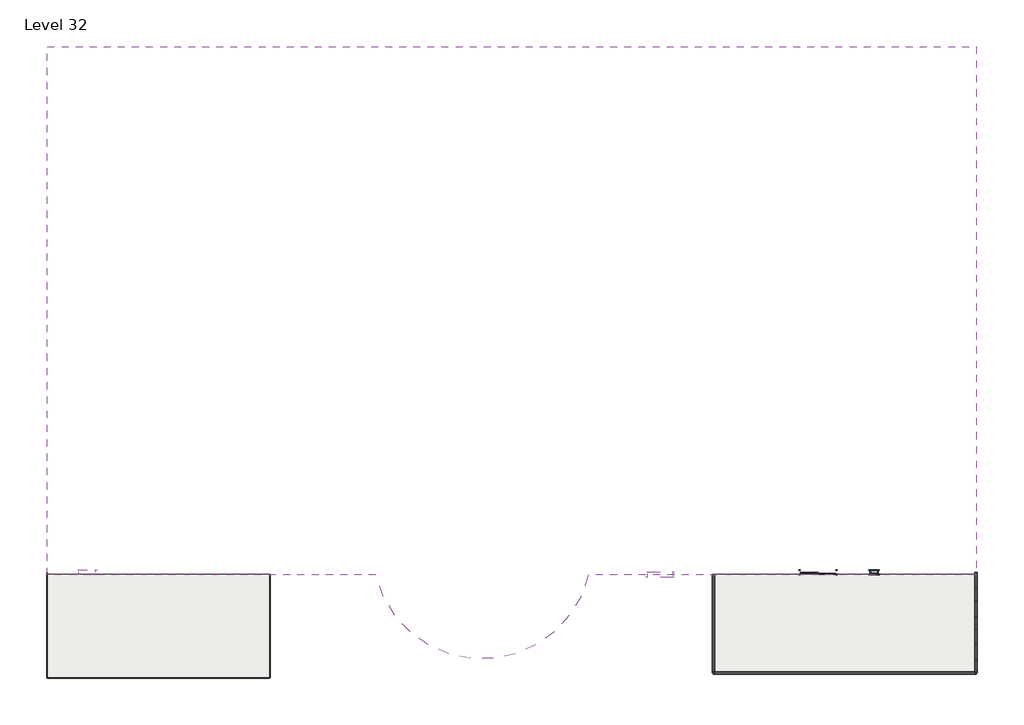
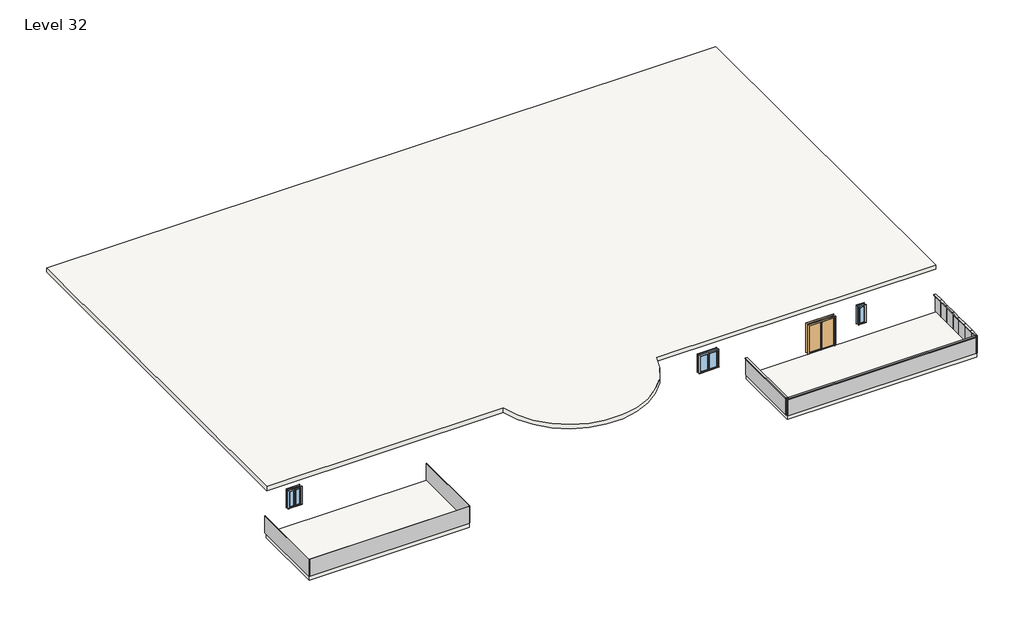
# One storey: 12 members, 12 plates, 3 slabs, 3 windows, 1 door.
"""IFC4 building model written with IfcOpenShell, lengths in millimetres."""

from ifc_helpers import new_model, si_unit, point, frame, frame_2d, origin, place, context, project, spatial, polyline, circle_curve, trimmed, segment, composite_curve, outline, extrude, transform, mapped, element, save
from components import door_076b30e0, member_bf9e663f, member_75074519, member_dd9ec6c9, member_47bfaf8a, member_aa870034, member_dcca090c, member_c1a40fae, member_a980948f, system_panel_glazed_64dbbd21, system_panel_glazed_febc6b86, system_panel_glazed_f269d4c8, system_panel_glazed_7af1c9c3, system_panel_glazed_5b6ac675, system_panel_glazed_8be6732c, system_panel_glazed_16eb27bd, system_panel_glazed_c55d8a5b, system_panel_glazed_6c4e9d17, system_panel_glazed_83eff035, window_a765b88f, window_bb17773d, window_0862ab64

model = new_model("IFC4")

# Units and contexts
model_context = context("Model", 3, world=origin())
ifc_project = project(units=[si_unit("LENGTHUNIT", "METRE", prefix="MILLI")], contexts=[model_context])

# Site, building, storey
site = spatial("IfcSite", under=ifc_project)
building = spatial("IfcBuilding", under=site)
storey = spatial("IfcBuildingStorey", under=building, Name="Level 32", Elevation=53340.0)

# Door
placement = place(None, origin())
door_shape = door_076b30e0(model_context)
element("IfcDoor", 1, ObjectType="Door-Double-Sliding : 68\" x 80\"", at=placement, inside=storey, context=model_context, shape_type="MappedRepresentation", body=[
    mapped(door_shape, transform((17768.214721, -12227.7237084, 53340.0), x_axis=(-1.0, 0.0, 0.0), y_axis=(0.0, -1.0, 0.0), z_axis=(0.0, 0.0, 1.0))),
])

# Members
member_shape = member_bf9e663f(model_context)
element("IfcMember", 2, ObjectType="Rectangular Mullion : 2.5\" x 5\" rectangular", at=placement, inside=storey, context=model_context, shape_type="MappedRepresentation", body=[
    mapped(member_shape, transform((12667.5594464, -12456.3237084, 54559.2), x_axis=(0.0, 0.0, 1.0), y_axis=(1.0, 0.0, 0.0), z_axis=(0.0, 1.0, 0.0))),
])
member_2_shape = member_75074519(model_context)
element("IfcMember", 3, ObjectType="Rectangular Mullion : 2.5\" x 5\" rectangular", at=placement, inside=storey, context=model_context, shape_type="MappedRepresentation", body=[
    mapped(member_2_shape, transform((12667.5594464, -17256.1078575, 54559.2), x_axis=(0.0, -1.0, 0.0), y_axis=(1.0, 0.0, 0.0), z_axis=(0.0, 0.0, 1.0))),
])
element("IfcMember", 4, ObjectType="Rectangular Mullion : 2.5\" x 5\" rectangular", at=placement, inside=storey, context=model_context, shape_type="MappedRepresentation", body=[
    mapped(member_2_shape, transform((25489.814721, -17256.1078575, 54559.2), x_axis=(1.0, 0.0, 0.0), y_axis=(0.0, 1.0, 0.0), z_axis=(0.0, 0.0, 1.0))),
])
member_3_shape = member_dd9ec6c9(model_context)
element("IfcMember", 5, ObjectType="Rectangular Mullion : 2.5\" x 5\" rectangular", at=placement, inside=storey, context=model_context, shape_type="MappedRepresentation", body=[
    mapped(member_3_shape, transform((12667.5594464, -17256.1078575, 54559.2), x_axis=(0.0, 0.0, 1.0), y_axis=(0.0, 1.0, 0.0), z_axis=(-1.0, 0.0, 0.0))),
])
member_4_shape = member_47bfaf8a(model_context)
element("IfcMember", 6, ObjectType="Rectangular Mullion : 2.5\" x 5\" rectangular", at=placement, inside=storey, context=model_context, shape_type="MappedRepresentation", body=[
    mapped(member_4_shape, transform((25489.814721, -15122.5078575, 54559.2), x_axis=(0.0, 0.0, 1.0), y_axis=(-1.0, 0.0, 0.0), z_axis=(0.0, -1.0, 0.0))),
])
member_5_shape = member_aa870034(model_context)
element("IfcMember", 7, ObjectType="Rectangular Mullion : 2.5\" x 5\" rectangular", at=placement, inside=storey, context=model_context, shape_type="MappedRepresentation", body=[
    mapped(member_5_shape, transform((25489.814721, -15884.5078575, 54559.2), x_axis=(0.0, 0.0, 1.0), y_axis=(-1.0, 0.0, 0.0), z_axis=(0.0, -1.0, 0.0))),
])
element("IfcMember", 8, ObjectType="Rectangular Mullion : 2.5\" x 5\" rectangular", at=placement, inside=storey, context=model_context, shape_type="MappedRepresentation", body=[
    mapped(member_5_shape, transform((25489.814721, -16646.5078575, 54559.2), x_axis=(0.0, 0.0, 1.0), y_axis=(-1.0, 0.0, 0.0), z_axis=(0.0, -1.0, 0.0))),
])
element("IfcMember", 9, ObjectType="Rectangular Mullion : 2.5\" x 5\" rectangular", at=placement, inside=storey, context=model_context, shape_type="MappedRepresentation", body=[
    mapped(member_2_shape, transform((25489.814721, -17256.1078575, 53340.0), x_axis=(0.0, -1.0, 0.0), y_axis=(-1.0, 0.0, 0.0), z_axis=(0.0, 0.0, -1.0))),
])
member_6_shape = member_dcca090c(model_context)
element("IfcMember", 10, ObjectType="Rectangular Mullion : 2.5\" x 5\" rectangular", at=placement, inside=storey, context=model_context, shape_type="MappedRepresentation", body=[
    mapped(member_6_shape, transform((25489.814721, -13046.6697457, 54559.2), x_axis=(0.0, 0.0, 1.0), y_axis=(-1.0, 0.0, 0.0), z_axis=(0.0, -1.0, 0.0))),
])
member_7_shape = member_c1a40fae(model_context)
element("IfcMember", 11, ObjectType="Rectangular Mullion : 2.5\" x 5\" rectangular", at=placement, inside=storey, context=model_context, shape_type="MappedRepresentation", body=[
    mapped(member_7_shape, transform((25489.814721, -14512.9078575, 54559.2), x_axis=(0.0, 0.0, 1.0), y_axis=(-1.0, 0.0, 0.0), z_axis=(0.0, -1.0, 0.0))),
])
element("IfcMember", 12, ObjectType="Rectangular Mullion : 2.5\" x 5\" rectangular", at=placement, inside=storey, context=model_context, shape_type="MappedRepresentation", body=[
    mapped(member_6_shape, transform((25489.814721, -13738.615783, 54559.2), x_axis=(0.0, 0.0, 1.0), y_axis=(-1.0, 0.0, 0.0), z_axis=(0.0, -1.0, 0.0))),
])
member_8_shape = member_a980948f(model_context)
element("IfcMember", 13, ObjectType="Rectangular Mullion : 2.5\" x 5\" rectangular", at=placement, inside=storey, context=model_context, shape_type="MappedRepresentation", body=[
    mapped(member_8_shape, transform((25489.814721, -17192.6078575, 54559.2), x_axis=(0.0, 0.0, 1.0), y_axis=(-1.0, 0.0, 0.0), z_axis=(0.0, -1.0, 0.0))),
])

# Plates
system_panel_glazed_shape = system_panel_glazed_64dbbd21(model_context)
element("IfcPlate", 14, ObjectType="System Panel : Glazed", at=placement, inside=storey, context=model_context, shape_type="MappedRepresentation", body=[
    mapped(system_panel_glazed_shape, transform((12667.5594464, -14824.465783, 53340.0), x_axis=(0.0, 1.0, 0.0), y_axis=(-1.0, 0.0, 0.0), z_axis=(0.0, 0.0, 1.0))),
])
system_panel_glazed_2_shape = system_panel_glazed_febc6b86(model_context)
element("IfcPlate", 15, ObjectType="System Panel : Glazed", at=placement, inside=storey, context=model_context, shape_type="MappedRepresentation", body=[
    mapped(system_panel_glazed_2_shape, transform((19046.9370837, -17256.1078575, 53340.0), x_axis=(-1.0, 0.0, 0.0), y_axis=(0.0, -1.0, 0.0), z_axis=(0.0, 0.0, 1.0))),
])
system_panel_glazed_3_shape = system_panel_glazed_f269d4c8(model_context)
element("IfcPlate", 16, ObjectType="System Panel : Glazed", at=placement, inside=storey, context=model_context, shape_type="MappedRepresentation", body=[
    mapped(system_panel_glazed_3_shape, transform((25489.814721, -16265.5078575, 53340.0), x_axis=(0.0, -1.0, 0.0), y_axis=(1.0, 0.0, 0.0), z_axis=(0.0, 0.0, 1.0))),
])
element("IfcPlate", 17, ObjectType="System Panel : Glazed", at=placement, inside=storey, context=model_context, shape_type="MappedRepresentation", body=[
    mapped(system_panel_glazed_3_shape, transform((25489.814721, -15503.5078575, 53340.0), x_axis=(0.0, -1.0, 0.0), y_axis=(1.0, 0.0, 0.0), z_axis=(0.0, 0.0, 1.0))),
])
system_panel_glazed_4_shape = system_panel_glazed_7af1c9c3(model_context)
element("IfcPlate", 18, ObjectType="System Panel : Glazed", at=placement, inside=storey, context=model_context, shape_type="MappedRepresentation", body=[
    mapped(system_panel_glazed_4_shape, transform((25489.814721, -14817.7078575, 53340.0), x_axis=(0.0, -1.0, 0.0), y_axis=(1.0, 0.0, 0.0), z_axis=(0.0, 0.0, 1.0))),
])
system_panel_glazed_5_shape = system_panel_glazed_5b6ac675(model_context)
element("IfcPlate", 19, ObjectType="System Panel : Glazed", at=placement, inside=storey, context=model_context, shape_type="MappedRepresentation", body=[
    mapped(system_panel_glazed_5_shape, transform((25489.814721, -12700.696727, 53340.0), x_axis=(0.0, -1.0, 0.0), y_axis=(1.0, 0.0, 0.0), z_axis=(0.0, 0.0, 1.0))),
])
element("IfcPlate", 20, ObjectType="System Panel : Glazed", at=placement, inside=storey, context=model_context, shape_type="MappedRepresentation", body=[
    mapped(system_panel_glazed_5_shape, transform((25489.814721, -13392.6427643, 53340.0), x_axis=(0.0, -1.0, 0.0), y_axis=(1.0, 0.0, 0.0), z_axis=(0.0, 0.0, 1.0))),
])
system_panel_glazed_6_shape = system_panel_glazed_8be6732c(model_context)
element("IfcPlate", 21, ObjectType="System Panel : Glazed", at=placement, inside=storey, context=model_context, shape_type="MappedRepresentation", body=[
    mapped(system_panel_glazed_6_shape, transform((25489.814721, -16919.5578575, 53340.0), x_axis=(0.0, -1.0, 0.0), y_axis=(1.0, 0.0, 0.0), z_axis=(0.0, 0.0, 1.0))),
])
system_panel_glazed_7_shape = system_panel_glazed_16eb27bd(model_context)
element("IfcPlate", 22, ObjectType="System Panel : Glazed", at=placement, inside=storey, context=model_context, shape_type="MappedRepresentation", body=[
    mapped(system_panel_glazed_7_shape, transform((25489.814721, -14125.7618202, 53340.0), x_axis=(0.0, -1.0, 0.0), y_axis=(1.0, 0.0, 0.0), z_axis=(0.0, 0.0, 1.0))),
])
system_panel_glazed_8_shape = system_panel_glazed_c55d8a5b(model_context)
element("IfcPlate", 23, ObjectType="System Panel : Glazed", at=placement, inside=storey, context=model_context, shape_type="MappedRepresentation", body=[
    mapped(system_panel_glazed_8_shape, transform((-9003.385279, -14970.9237084, 53340.0), x_axis=(0.0, -1.0, 0.0), y_axis=(1.0, 0.0, 0.0), z_axis=(0.0, 0.0, 1.0))),
])
system_panel_glazed_9_shape = system_panel_glazed_6c4e9d17(model_context)
element("IfcPlate", 24, ObjectType="System Panel : Glazed", at=placement, inside=storey, context=model_context, shape_type="MappedRepresentation", body=[
    mapped(system_panel_glazed_9_shape, transform((-14413.585279, -17485.5237084, 53340.0), x_axis=(-1.0, 0.0, 0.0), y_axis=(0.0, -1.0, 0.0), z_axis=(0.0, 0.0, 1.0))),
])
system_panel_glazed_10_shape = system_panel_glazed_83eff035(model_context)
element("IfcPlate", 25, ObjectType="System Panel : Glazed", at=placement, inside=storey, context=model_context, shape_type="MappedRepresentation", body=[
    mapped(system_panel_glazed_10_shape, transform((-19823.785279, -14920.1237084, 53340.0), x_axis=(0.0, 1.0, 0.0), y_axis=(-1.0, 0.0, 0.0), z_axis=(0.0, 0.0, 1.0))),
])

# Slabs
element("IfcSlab", 26, ObjectType="Generic - 12\"", at=placement, inside=storey, context=model_context, shape_type="SweptSolid", body=[
    extrude(outline(composite_curve([segment(polyline([(25489.814721, 13324.8600062), (25489.814721, -12481.5399938), (6571.5594464, -12481.5399938)]), True, "CONTINUOUS"), segment(trimmed(circle_curve(frame_2d((1385.214721, -11250.9069525)), 5330.3498284), [point((6571.5594464, -12481.5399938))], [point((-3801.1300045, -12481.5399938))], False, "CARTESIAN"), True, "CONTINUOUS"), segment(polyline([(-3801.1300045, -12481.5399938), (-19823.785279, -12481.5399938), (-19823.785279, 13324.8600062), (25489.814721, 13324.8600062)]), True, "CONTINUOUS")], self_intersect=False)), frame((0.0, 0.0, 56425.3367162), z_axis=(0.0, 0.0, 1.0), x_axis=(1.0, 0.0, 0.0)), (0.0, 0.0, 1.0), 304.8),
])
element("IfcSlab", 27, ObjectType="Generic - 12\"", at=placement, inside=storey, context=model_context, shape_type="SweptSolid", body=[
    extrude(outline(polyline([(25489.814721, -12456.3237084), (25489.814721, -17256.1078575), (12667.5594464, -17256.1078575), (12667.5594464, -12456.3237084), (25489.814721, -12456.3237084)])), frame((0.0, 0.0, 53035.2), z_axis=(0.0, 0.0, 1.0), x_axis=(1.0, 0.0, 0.0)), (0.0, 0.0, 1.0), 304.8),
])
element("IfcSlab", 28, ObjectType="Generic - 12\"", at=placement, inside=storey, context=model_context, shape_type="SweptSolid", body=[
    extrude(outline(polyline([(-9003.385279, -12456.3237084), (-9003.385279, -17485.5237084), (-19823.785279, -17485.5237084), (-19823.785279, -12456.3237084), (-9003.385279, -12456.3237084)])), frame((0.0, 0.0, 53035.2), z_axis=(0.0, 0.0, 1.0), x_axis=(1.0, 0.0, 0.0)), (0.0, 0.0, 1.0), 304.8),
])

# Windows
window_shape = window_a765b88f(model_context)
element("IfcWindow", 29, ObjectType="Awning with Trim : 16\" x 48\"", at=placement, inside=storey, context=model_context, shape_type="MappedRepresentation", body=[
    mapped(window_shape, transform((20511.414721, -12354.7237084, 53340.0), x_axis=(-1.0, 0.0, 0.0), y_axis=(0.0, -1.0, 0.0), z_axis=(0.0, 0.0, 1.0))),
])
window_2_shape = window_bb17773d(model_context)
element("IfcWindow", 30, ObjectType="Casement Dbl with Trim : 32\" x 48\"", at=placement, inside=storey, context=model_context, shape_type="MappedRepresentation", body=[
    mapped(window_2_shape, transform((-17893.385279, -12335.6737084, 53689.214928), x_axis=(-1.0, 0.0, 0.0), y_axis=(0.0, -1.0, 0.0), z_axis=(0.0, 0.0, 1.0))),
])
window_3_shape = window_0862ab64(model_context)
element("IfcWindow", 31, ObjectType="Casement Dbl with Trim : 48\" x 48\"", at=placement, inside=storey, context=model_context, shape_type="MappedRepresentation", body=[
    mapped(window_3_shape, transform((10076.7594464, -12437.2737084, 53715.539368), x_axis=(-1.0, 0.0, 0.0), y_axis=(0.0, -1.0, 0.0), z_axis=(0.0, 0.0, 1.0))),
])

save(model, "model.ifc")

# Revit data of these elements
# Type "Door-Double-Sliding : 68\" x 80\""
#   Type Mark = "10"
#   Construction Type Id = "opn-d45"
#   Assembly Code = "C1020"
#   Analytic Construction = "Wood frame, double glass door "
#   Thickness = 0' - 2"
#   Thermal Resistance (R) = 1.8150 (h·ft²·°F)/BTU
#   Heat Transfer Coefficient (U) = 0.5510 BTU/(h·ft²·°F)
#   Height = 6' - 8"
#   Rail Width = 0' - 2"
#   Stiles = 0' - 2"
#   Trim Projection Ext = 0' - 1"
#   Trim Projection Int = 0' - 1"
#   Trim Width = 0' - 3"
#   Width = 5' - 8"
#   Define Thermal Properties by = 1
#   Glazing = Glass
#   Panel Material = Wood - Birch - Solid Stained Light Low Gloss
#   Trim Material = Paint - Sienna
#   Visual Light Transmittance = 0
#   Solar Heat Gain Coefficient = 0
#   Function = (empty or 0)
#   Wall Closure = (empty or 0)
# Type "Rectangular Mullion : 2.5\" x 5\" rectangular"
#   built-in parameter 1007304 = 0.416667 (stored number, unit not read)
#   built-in parameter 1007301 = 0.104167 (stored number, unit not read)
#   built-in parameter 1007300 = 0.104167 (stored number, unit not read)
# Type "System Panel : Glazed"
#   Construction Type Id = "GSP4R"
#   Analytic Construction = "1/8 in Pilkington single glazing"
#   Visual Light Transmittance = 0.9
#   Solar Heat Gain Coefficient = 0.86
#   Heat Transfer Coefficient (U) = 1.18115 BTU/(h·ft²·°F)
# Type "Generic - 12\""
#   Assembly Code = "B1010"
#   Function = 0
#   Layers, outside or top first: 1' - 0" no material (function 1)
# Type "Awning with Trim : 16\" x 48\""
#   Type Mark = "14"
#   Construction Type Id = "GSP4R"
#   Assembly Code = "B2020100"
#   Analytic Construction = "1/8 in Pilkington single glazing"
#   Visual Light Transmittance = 0.9
#   Solar Heat Gain Coefficient = 0.78
#   Heat Transfer Coefficient (U) = 0.6496 BTU/(h·ft²·°F)
#   Height = 4' - 0"
#   Default Sill Height = 3' - 0"
#   Trim Projection - Ext. = 0' - 0 1/2"
#   Trim Projection - Int. = 0' - 0 3/4"
#   Trim Width - Exterior = 0' - 3 1/2"
#   Trim Width - Interior = 0' - 3 1/2"
#   Width = 1' - 4"
#   Window Inset = 0' - 0 3/4"
#   Define Thermal Properties by = 1
#   Glass Pane Material = Glass
#   Sash Material = Sash
#   Trim Exterior Material = Trim
#   Trim Interior Material = Trim
#   Wall Closure = (empty or 0)
# Type "Casement Dbl with Trim : 32\" x 48\""
#   Type Mark = "36"
#   Construction Type Id = "GSP4R"
#   Assembly Code = "B2020100"
#   Analytic Construction = "1/8 in Pilkington single glazing"
#   Visual Light Transmittance = 0.9
#   Solar Heat Gain Coefficient = 0.78
#   Heat Transfer Coefficient (U) = 0.6496 BTU/(h·ft²·°F)
#   Height = 4' - 0"
#   Default Sill Height = 3' - 0"
#   Trim Projection - Ext. = 0' - 0 1/2"
#   Trim Projection - Int. = 0' - 0 3/4"
#   Trim Width - Exterior = 0' - 3 1/2"
#   Trim Width - Interior = 0' - 3 1/2"
#   Width = 2' - 8"
#   Window Inset = 0' - 0 3/4"
#   Define Thermal Properties by = 1
#   Glass Pane Material = Glass
#   Sash Material = Sash
#   Trim Exterior Material = Trim
#   Trim Interior Material = Trim
#   Wall Closure = (empty or 0)
# Type "Casement Dbl with Trim : 48\" x 48\""
#   Type Mark = "34"
#   Construction Type Id = "GSP4R"
#   Assembly Code = "B2020100"
#   Analytic Construction = "1/8 in Pilkington single glazing"
#   Visual Light Transmittance = 0.9
#   Solar Heat Gain Coefficient = 0.78
#   Heat Transfer Coefficient (U) = 0.6496 BTU/(h·ft²·°F)
#   Height = 4' - 0"
#   Default Sill Height = 3' - 0"
#   Trim Projection - Ext. = 0' - 0 1/2"
#   Trim Projection - Int. = 0' - 0 3/4"
#   Trim Width - Exterior = 0' - 3 1/2"
#   Trim Width - Interior = 0' - 3 1/2"
#   Width = 4' - 0"
#   Window Inset = 0' - 0 3/4"
#   Define Thermal Properties by = 1
#   Glass Pane Material = Glass
#   Sash Material = Sash
#   Trim Exterior Material = Trim
#   Trim Interior Material = Trim
#   Wall Closure = (empty or 0)
# Element 1 (IfcDoor, "Door-Double-Sliding : 68\" x 80\"")
#   Phase Created = New Construction
#   Materials on its faces: "Paint - Sienna", "Wood - Birch - Solid Stained Light Low Gloss", "Glass"
# Elements 2, 3, 4, 5, 6, 7, 8, 9, 10, 11, 12, 13 (IfcMember, "Rectangular Mullion : 2.5\" x 5\" rectangular")
#   Phase Created = New Construction
#   Materials on its faces: "Aluminum"
# Elements 14, 15, 16, 17, 18, 19, 20, 21, 22, 23, 24, 25 (IfcPlate, "System Panel : Glazed")
#   Phase Created = New Construction
#   Materials on its faces: "Glass"
# Element 26 (IfcSlab, "Generic - 12\"")
#   Height Offset From Level = 11' - 1.46995"
#   Phase Created = New Construction
#   Materials on its faces: "Default Floor"
# Elements 27, 28 (IfcSlab, "Generic - 12\"")
#   Height Offset From Level = 0' - 0"
#   Phase Created = New Construction
#   Materials on its faces: "Default Floor"
# Element 29 (IfcWindow, "Awning with Trim : 16\" x 48\"")
#   Mark = "52"
#   Phase Created = New Construction
#   Materials on its faces: "Sash", "Trim", "Glass"
# Element 30 (IfcWindow, "Casement Dbl with Trim : 32\" x 48\"")
#   Mark = "35"
#   Phase Created = New Construction
#   Materials on its faces: "Sash", "Trim", "Glass"
# Element 31 (IfcWindow, "Casement Dbl with Trim : 48\" x 48\"")
#   Mark = "1"
#   Phase Created = New Construction
#   Materials on its faces: "Sash", "Trim", "Glass"
# Materials
#   "Glass": class "Glass", colour RGB 0 128 192, transparency 0.75, Description = "Soda Lime Glass", Cost = 0
#   "Wood - Birch - Solid Stained Light Low Gloss": class "Wood", colour RGB 210 159 95, transparency 0, Cost = 0
#   "Paint - Sienna": colour RGB 118 70 51, transparency 0, Cost = 0
#   "Sash": class "Wood", colour RGB 224 178 126, transparency 0
#   "Trim": class "Wood", colour RGB 224 178 126, transparency 0
#   "Aluminum": class "Metal", colour RGB 247 247 247, transparency 0, Description = "Aluminum 6061", Cost = 0
#   "Default Floor": colour RGB 128 128 128, transparency 0
